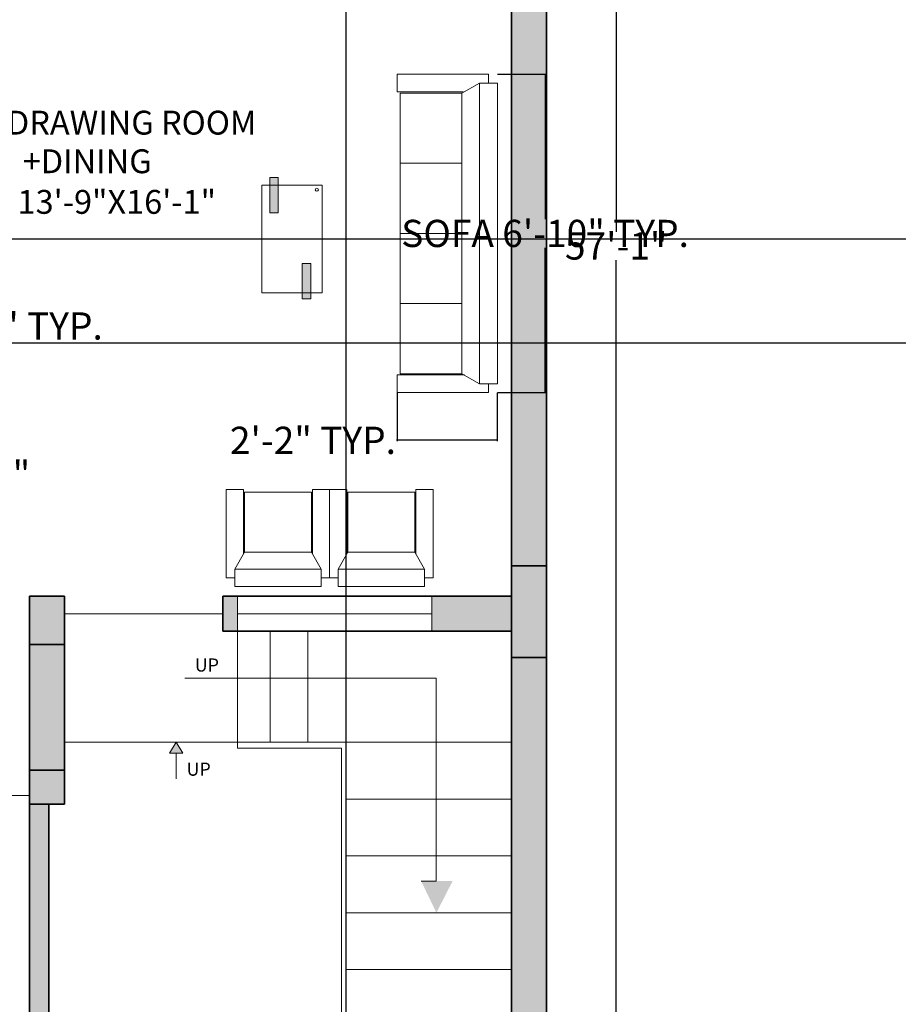
# Model space of a CAD drawing. Units: inches. Extents: x -17 to 892, y -721 to 172.
# Tile 3 of 11: x 212 to 438, y -462 to -209. Entities that reach past the tile are written whole.
import ezdxf

# ---------------------------------------------------------------- set-up
doc = ezdxf.new("R2010")
doc.units = ezdxf.units.IN
doc.header["$MEASUREMENT"] = 0
doc.layers.get('0').update_dxf_attribs({"color": 14})
for name, color, linetype, lineweight in [('A-ANNO-DIMS', 2, 'Continuous', 18), ('A-ANNO-SYMB', 7, 'Continuous', 18), ('A-AREA-IDEN', 7, 'Continuous', 18), ('A-COLS', 252, 'Continuous', 35), ('A-FLOR-STRS', 8, 'Continuous', 18), ('A-WALL-PATT', 14, 'Continuous', 13), ('doors', 4, 'Continuous', 18), ('furniture', 252, 'Continuous', 18), ('walls', 252, 'Continuous', 35), ('windows', 161, 'Continuous', 18)]:
    doc.layers.add(name, color=color, linetype=linetype, lineweight=lineweight)
doc.layers.add('A-COLS-PATT', color=254, linetype='Continuous', lineweight=13, true_color=0xd7ebd2)
doc.styles.get("Standard").update_dxf_attribs({"font": 'arial.ttf'})
doc.dimstyles.get("Standard").update_dxf_attribs({"dimtxt": 7, "dimasz": 0.18, "dimexe": 0.18, "dimexo": 0.0625, "dimgap": 0.09, "dimtad": 0, "dimtih": 1, "dimtoh": 1, "dimzin": 0, "dimdsep": 46, "dimlunit": 3, "dimtxsty": 'Standard', "dimcen": 0.09, "dimadec": 0, "dimazin": 0, "dimtfac": 1, "dimtofl": 0, "dimtmove": 0, "dimatfit": 3, "dimfxl": 1, "dimtolj": 1, "dimtzin": 0, "dimarcsym": 0})

# ---------------------------------------------------------------- blocks, each defined once
blk = doc.blocks.new('FABRIC SOFA 1S')
at = {"layer": 'furniture'}
for p, q in [((3, 18.12), (34, 18.12)), ((3, 15.12), (3, 18.12)), ((34, 12.12), (34, 18.12)), ((0, -15.12), (0, 15.12)), ((6, 15.12), (0, 15.12)), ((6, -15.12), (6, 15.12)), ((12, 11.75), (6, 15.12)), ((11.33, 12.12), (34, 12.12)), ((6, -15.12), (12, -11.75)), ((11.33, -12.12), (34, -12.12)), ((34, -12.12), (34, -18.12)), ((6, -15.12), (0, -15.12)), ((3, -18.12), (3, -15.12)), ((3, -18.12), (34, -18.12))]:
    blk.add_line(p, q, dxfattribs=at)
blk.add_lwpolyline([(12, -11.75), (12, 11.75), (33, 11.75), (33, -11.75)], close=True, dxfattribs=at)
blk = doc.blocks.new('FABRIC SOFA 4S')
at = {"layer": 'furniture'}
for p, q in [((3, 54), (34, 54)), ((3, 51), (3, 54)), ((34, 48), (34, 54)), ((0, -51), (0, 51)), ((6, 51), (0, 51)), ((6, -51), (6, 51)), ((12, 47.63), (6, 51)), ((11.14, 48), (34, 48)), ((33, 23.81), (12, 23.81)), ((33, 0), (12, 0)), ((33, -23.81), (12, -23.81)), ((6, -51), (12, -47.63)), ((11.54, -48), (34, -48)), ((34, -48), (34, -54)), ((6, -51), (0, -51)), ((3, -54), (3, -51)), ((3, -54), (34, -54))]:
    blk.add_line(p, q, dxfattribs=at)
blk.add_lwpolyline([(12, -47.63), (12, 47.63), (33, 47.63), (33, -47.63)], close=True, dxfattribs=at)
blk = doc.blocks.new('*D16')
at = {"layer": 'A-ANNO-DIMS', "color": 0, "lineweight": -2, "transparency": 16777216}
for p, q in [((364.49, 89.9), (365.24, 89.9)), ((365.06, 89.72), (365.06, -263.08)), ((365.06, -623.21), (365.06, -270.41)), ((364.49, -623.39), (365.24, -623.39))]:
    blk.add_line(p, q, dxfattribs=at)
at = {"layer": 'A-ANNO-DIMS', "color": 0, "lineweight": 100, "transparency": 16777216}
for points in [[(365.03, 89.72), (365.09, 89.72), (365.06, 89.9)], [(365.03, -623.21), (365.09, -623.21), (365.06, -623.39)]]:
    blk.add_solid(points, dxfattribs=at)
at = {"layer": 'Defpoints', "color": 0, "lineweight": 100, "transparency": 16777216}
for p in [(364.43, 89.9), (364.43, -623.39), (365.06, -623.39)]:
    blk.add_point(p, dxfattribs=at)
at = {"layer": 'A-ANNO-DIMS', "color": 0, "transparency": 16777216, "insert": (365.06, -266.74), "char_height": 7, "attachment_point": 5}
blk.add_mtext('\\A1;57\'-1"', dxfattribs=at)
blk = doc.blocks.new('TABLE-COCKTAIL')
h = blk.add_hatch(color=256)
h.dxf.hatch_style = 1
h.paths.add_polyline_path([(4.23, 29.31), (2.04, 29.31), (2.04, 22.19), (4.23, 22.19)])
h.paths.add_polyline_path([(4.23, 31.28), (2.04, 31.28), (2.04, 29.31), (4.23, 29.31)])
h.paths.add_polyline_path([(12.58, 9.09), (10.39, 9.09), (10.39, 1.62), (12.58, 1.62)])
h.paths.add_polyline_path([(12.58, 1.62), (10.39, 1.62), (10.39, 0), (12.58, 0)])
for p, q in [((2.04, 31.28), (4.23, 31.28)), ((2.04, 22.19), (2.04, 31.28)), ((4.23, 31.28), (4.23, 22.19)), ((0, 29.31), (0, 1.62)), ((15.53, 29.31), (0, 29.31)), ((15.53, 1.62), (15.53, 29.31)), ((4.23, 22.19), (2.04, 22.19)), ((10.39, 9.09), (12.58, 9.09)), ((10.39, 0), (10.39, 9.09)), ((12.58, 9.09), (12.58, 0)), ((0, 1.62), (15.53, 1.62)), ((12.58, 0), (10.39, 0))]:
    blk.add_line(p, q)
blk.add_circle((14.17, 28.1), 0.401)
blk = doc.blocks.new('STAIR-DIRECTION')
h = blk.add_hatch(color=256)
h.dxf.hatch_style = 1
h.paths.add_polyline_path([(64.68, 8.16), (60.81, 8.16), (64.68, 0.16)])
h.paths.add_polyline_path([(68.92, 8.16), (64.68, 8.16), (64.68, 0.16), (64.75, 0)])
for p, q in [((0, 60.33), (64.68, 60.33)), ((64.68, 60.33), (64.68, 8.16)), ((64.68, 8.16), (60.81, 8.16))]:
    blk.add_line(p, q)
blk = doc.blocks.new('*D44')
at = {"layer": 'A-ANNO-DIMS', "color": 0, "lineweight": -2, "transparency": 16777216}
for p, q in [((334.53, -222.56), (346.93, -222.56)), ((346.75, -222.74), (346.75, -259.8)), ((346.75, -304.28), (346.75, -267.22)), ((334.53, -304.46), (346.93, -304.46))]:
    blk.add_line(p, q, dxfattribs=at)
at = {"layer": 'A-ANNO-DIMS', "color": 0, "lineweight": 100, "transparency": 16777216}
for points in [[(346.72, -222.74), (346.78, -222.74), (346.75, -222.56)], [(346.72, -304.28), (346.78, -304.28), (346.75, -304.46)]]:
    blk.add_solid(points, dxfattribs=at)
at = {"layer": 'Defpoints', "color": 0, "lineweight": 100, "transparency": 16777216}
for p in [(334.46, -222.56), (334.46, -304.46), (346.75, -304.46)]:
    blk.add_point(p, dxfattribs=at)
at = {"layer": 'A-ANNO-DIMS', "color": 0, "transparency": 16777216, "insert": (346.75, -263.51), "char_height": 7, "attachment_point": 5}
blk.add_mtext('\\A1;SOFA 6\'-10" TYP.', dxfattribs=at)
blk = doc.blocks.new('*D45')
at = {"layer": 'A-ANNO-DIMS', "color": 0, "lineweight": -2, "transparency": 16777216}
for p, q in [((308.68, -304.52), (308.68, -316.93)), ((334.46, -304.52), (334.46, -316.93)), ((308.68, -316.75), (308.5, -316.75)), ((334.28, -316.75), (308.86, -316.75))]:
    blk.add_line(p, q, dxfattribs=at)
at = {"layer": 'A-ANNO-DIMS', "color": 0, "lineweight": 100, "transparency": 16777216}
for points in [[(308.86, -316.72), (308.86, -316.78), (308.68, -316.75)], [(334.28, -316.72), (334.28, -316.78), (334.46, -316.75)]]:
    blk.add_solid(points, dxfattribs=at)
at = {"layer": 'Defpoints', "color": 0, "lineweight": 100, "transparency": 16777216}
for p in [(308.68, -304.46), (334.46, -304.46), (308.68, -316.75)]:
    blk.add_point(p, dxfattribs=at)
at = {"layer": 'A-ANNO-DIMS', "color": 0, "transparency": 16777216, "insert": (287.02, -316.75), "char_height": 7, "attachment_point": 5}
blk.add_mtext('\\A1;2\'-2" TYP.', dxfattribs=at)
blk = doc.blocks.new('*D51')
at = {"layer": 'A-ANNO-DIMS', "color": 0, "lineweight": -2, "transparency": 16777216}
for p, q in [((170.93, -291.56), (170.93, -287.14)), ((171.11, -287.32), (173.4, -287.32)), ((173.58, -291.56), (173.58, -287.14)), ((173.58, -287.32), (173.76, -287.32))]:
    blk.add_line(p, q, dxfattribs=at)
at = {"layer": 'A-ANNO-DIMS', "color": 0, "lineweight": 100, "transparency": 16777216}
for points in [[(171.11, -287.29), (171.11, -287.35), (170.93, -287.32)], [(173.4, -287.29), (173.4, -287.35), (173.58, -287.32)]]:
    blk.add_solid(points, dxfattribs=at)
at = {"layer": 'Defpoints', "color": 0, "lineweight": 100, "transparency": 16777216}
for p in [(173.58, -287.32), (170.93, -291.63), (173.58, -291.63)]:
    blk.add_point(p, dxfattribs=at)
at = {"layer": 'A-ANNO-DIMS', "color": 0, "transparency": 16777216, "insert": (203.34, -287.32), "char_height": 7, "attachment_point": 5}
blk.add_mtext('\\A1;0\'-2 1/2" TYP.', dxfattribs=at)
blk = doc.blocks.new('*D54')
at = {"layer": 'A-ANNO-DIMS', "color": 0, "lineweight": -2, "transparency": 16777216}
for p, q in [((133.16, -328.67), (133.16, -325.31)), ((133.34, -325.49), (154.58, -325.49)), ((154.76, -328.67), (154.76, -325.31)), ((154.76, -325.49), (154.94, -325.49))]:
    blk.add_line(p, q, dxfattribs=at)
at = {"layer": 'A-ANNO-DIMS', "color": 0, "lineweight": 100, "transparency": 16777216}
for points in [[(133.34, -325.46), (133.34, -325.52), (133.16, -325.49)], [(154.58, -325.46), (154.58, -325.52), (154.76, -325.49)]]:
    blk.add_solid(points, dxfattribs=at)
at = {"layer": 'Defpoints', "color": 0, "lineweight": 100, "transparency": 16777216}
for p in [(154.76, -325.49), (133.16, -328.73), (154.76, -328.73)]:
    blk.add_point(p, dxfattribs=at)
at = {"layer": 'A-ANNO-DIMS', "color": 0, "transparency": 16777216, "insert": (184.26, -325.49), "char_height": 7, "attachment_point": 5}
blk.add_mtext('\\A1;HOB 1\'-9 1/2"', dxfattribs=at)
blk = doc.blocks.new('*D61')
at = {"layer": 'A-ANNO-DIMS', "color": 0, "lineweight": -2, "transparency": 16777216}
for p, q in [((170.99, -264.92), (841.36, -264.92)), ((841.18, -265.1), (841.18, -274.56)), ((841.18, -291.45), (841.18, -281.98)), ((170.99, -291.63), (841.36, -291.63))]:
    blk.add_line(p, q, dxfattribs=at)
at = {"layer": 'A-ANNO-DIMS', "color": 0, "lineweight": 100, "transparency": 16777216}
for points in [[(841.15, -265.1), (841.21, -265.1), (841.18, -264.92)], [(841.15, -291.45), (841.21, -291.45), (841.18, -291.63)]]:
    blk.add_solid(points, dxfattribs=at)
at = {"layer": 'Defpoints', "color": 0, "lineweight": 100, "transparency": 16777216}
for p in [(170.93, -264.92), (170.93, -291.63), (841.18, -291.63)]:
    blk.add_point(p, dxfattribs=at)
at = {"layer": 'A-ANNO-DIMS', "color": 0, "transparency": 16777216, "insert": (841.18, -278.27), "char_height": 7, "attachment_point": 5}
blk.add_mtext('\\A1;2\'-2 1/2"', dxfattribs=at)
blk = doc.blocks.new('*D63')
at = {"layer": 'A-ANNO-DIMS', "color": 0, "lineweight": -2, "transparency": 16777216}
for p, q in [((295.55, -619.99), (295.55, 161.84)), ((295.73, 161.66), (299.27, 161.66)), ((337.9, 161.66), (334.36, 161.66)), ((338.08, -619.99), (338.08, 161.84))]:
    blk.add_line(p, q, dxfattribs=at)
at = {"layer": 'A-ANNO-DIMS', "color": 0, "lineweight": 100, "transparency": 16777216}
for points in [[(295.73, 161.69), (295.73, 161.63), (295.55, 161.66)], [(337.9, 161.69), (337.9, 161.63), (338.08, 161.66)]]:
    blk.add_solid(points, dxfattribs=at)
at = {"layer": 'Defpoints', "color": 0, "lineweight": 100, "transparency": 16777216}
for p in [(338.08, 161.66), (295.55, -620.06), (338.08, -620.06)]:
    blk.add_point(p, dxfattribs=at)
at = {"layer": 'A-ANNO-DIMS', "color": 0, "transparency": 16777216, "insert": (316.82, 161.66), "char_height": 7, "attachment_point": 5}
blk.add_mtext('\\A1;3\'-6 1/2"', dxfattribs=at)

msp = doc.modelspace()

# ---------------------------------------------------------------- hatches: boundary and pattern name
at = {"layer": 'A-ANNO-SYMB'}
h = msp.add_hatch(color=256, dxfattribs=at)
h.dxf.hatch_style = 1
h.paths.add_polyline_path([(251.822, -394.434), (250.105, -397.283), (251.822, -397.283), (253.554, -397.283)])
at = {"layer": 'A-COLS-PATT'}
h = msp.add_hatch(color=256, dxfattribs=at)
h.dxf.hatch_style = 1
h.paths.add_polyline_path([(92.084, 61.611), (83.084, 61.611), (83.084, 43.692), (92.084, 43.692)])
h.paths.add_polyline_path([(347.084, 61.611), (338.084, 61.611), (338.084, 43.692), (347.084, 43.692)])
h.paths.add_polyline_path([(222.053, 61.611), (209.95, 61.611), (209.95, 52.611), (222.053, 52.611)])
h.paths.add_polyline_path([(284.798, 61.611), (274.584, 61.611), (274.584, 52.611), (284.798, 52.611)])
h.paths.add_polyline_path([(223.084, -106.389), (214.084, -106.389), (214.084, -119.959), (223.084, -119.959)])
h.paths.add_polyline_path([(347.084, -148.653), (338.084, -148.653), (338.084, -172.24), (347.084, -172.24)])
h.paths.add_polyline_path([(92.084, -102.402), (83.084, -102.402), (83.084, -119.959), (92.084, -119.959)])
h.paths.add_polyline_path([(92.084, -205.889), (83.084, -205.889), (83.084, -216.319), (92.084, -216.319)])
h.paths.add_polyline_path([(347.084, -349.073), (338.084, -349.073), (338.084, -372.66), (347.084, -372.66)])
h.paths.add_polyline_path([(347.084, -610.134), (338.084, -610.134), (338.084, -614.389), (338.084, -623.342), (347.084, -623.342)])
h.paths.add_polyline_path([(221.166, -610.357), (214.084, -610.357), (214.084, -623.389), (219.084, -623.389), (221.166, -623.389), (221.166, -621.723)])
h.paths.add_polyline_path([(90.166, -610.357), (83.084, -610.357), (83.084, -623.389), (90.166, -623.389)])
h.paths.add_polyline_path([(223.084, -401.64), (214.084, -401.64), (214.084, -410.389), (223.084, -410.389)])
h.paths.add_polyline_path([(223.084, -356.889), (214.084, -356.889), (214.084, -369.273), (223.084, -369.273)])
h.paths.add_polyline_path([(92.084, -398.492), (83.084, -398.492), (83.084, -410.389), (92.084, -410.389)])
h.paths.add_polyline_path([(92.084, -348.918), (83.084, -348.918), (83.084, -360.706), (92.084, -360.706)])
at = {"layer": 'A-WALL-PATT'}
h = msp.add_hatch(color=256, dxfattribs=at)
h.dxf.hatch_style = 1
h.paths.add_polyline_path([(111.26, 61.611), (92.084, 61.611), (92.084, 52.611), (111.26, 52.611)])
h.paths.add_polyline_path([(209.95, 61.611), (179.154, 61.611), (179.154, 52.611), (209.95, 52.611)])
h.paths.add_polyline_path([(338.084, 61.611), (284.798, 61.611), (284.798, 52.611), (338.084, 52.611)])
h.paths.add_polyline_path([(279.084, 23.861), (274.584, 23.861), (274.584, -0.389), (279.084, -0.389)])
h.paths.add_polyline_path([(279.084, 52.611), (274.584, 52.611), (274.584, 46.881), (276.834, 46.881), (279.084, 46.881)])
h.paths.add_polyline_path([(279.084, -0.389), (274.584, -0.389), (274.584, -4.889), (279.084, -4.889)])
h.paths.add_polyline_path([(304.22, -0.389), (279.084, -0.389), (279.084, -4.889), (304.22, -4.889)])
h.paths.add_polyline_path([(347.084, 43.692), (338.084, 43.692), (338.084, -148.653), (347.084, -148.653)])
h.paths.add_polyline_path([(338.084, -154.889), (264.103, -154.889), (264.103, -163.889), (338.084, -163.889)])
h.paths.add_polyline_path([(223.084, -119.959), (214.084, -119.959), (214.084, -163.889), (223.084, -163.889)])
h.paths.add_polyline_path([(218.584, 52.611), (214.084, 52.611), (214.084, -106.389), (218.584, -106.389)])
h.paths.add_polyline_path([(92.084, -8.943), (83.084, -8.943), (83.084, -49.69), (87.584, -49.69), (92.084, -49.69)])
h.paths.add_polyline_path([(92.084, 43.692), (83.084, 43.692), (83.084, 33.018), (87.584, 33.018), (92.084, 33.018)])
h.paths.add_polyline_path([(92.084, -91.651), (83.084, -91.651), (83.084, -102.402), (92.084, -102.402)])
h.paths.add_polyline_path([(92.084, -119.959), (83.084, -119.959), (83.084, -151.855), (87.584, -151.855), (92.084, -151.855)])
h.paths.add_polyline_path([(173.584, -108.639), (173.584, -106.389), (173.084, -106.389), (92.084, -106.389), (92.084, -110.889), (169.084, -110.889), (169.084, -176.029), (173.584, -176.029)])
h.paths.add_polyline_path([(92.084, -185.221), (83.084, -185.221), (83.084, -205.889), (92.084, -205.889)])
h.paths.add_polyline_path([(92.084, -216.319), (83.084, -216.319), (83.084, -259.015), (87.584, -259.015), (92.084, -259.015)])
h.paths.add_polyline_path([(173.584, -205.889), (92.084, -205.889), (92.084, -210.389), (169.084, -210.389), (169.084, -236.193), (173.584, -236.193)])
h.paths.add_polyline_path([(92.084, -300.976), (83.084, -300.976), (83.084, -348.918), (92.084, -348.918)])
h.paths.add_polyline_path([(87.584, -410.389), (83.084, -410.389), (83.084, -610.357), (87.584, -610.357)])
h.paths.add_polyline_path([(115.523, -614.389), (90.166, -614.389), (90.166, -623.389), (115.523, -623.389)])
h.paths.add_polyline_path([(214.084, -614.389), (174.149, -614.389), (174.149, -623.389), (214.084, -623.389)])
h.paths.add_polyline_path([(219.084, -410.389), (214.084, -410.389), (214.084, -610.357), (219.084, -610.357)])
h.paths.add_polyline_path([(347.084, -372.66), (338.084, -372.66), (338.084, -610.134), (347.084, -610.134)])
h.paths.add_polyline_path([(347.084, -172.24), (338.084, -172.24), (338.084, -349.073), (347.084, -349.073)])
h.paths.add_polyline_path([(338.084, -356.889), (317.618, -356.889), (317.618, -365.889), (338.084, -365.889)])
h.paths.add_polyline_path([(267.632, -356.889), (263.828, -356.889), (263.828, -365.889), (267.632, -365.889)])
h.paths.add_polyline_path([(223.084, -369.273), (214.084, -369.273), (214.084, -401.64), (223.084, -401.64)])

# ---------------------------------------------------------------- linework, layer by layer
at = {"layer": 'A-ANNO-SYMB'}
for p, q in [((251.822, -394.434), (250.105, -397.283)), ((253.554, -397.283), (251.822, -394.434)), ((250.105, -397.283), (251.822, -397.283)), ((251.822, -397.283), (253.554, -397.283)), ((251.822, -397.283), (251.822, -403.838))]:
    msp.add_line(p, q, dxfattribs=at)
at = {"layer": 'A-COLS'}
for p, q in [((338.084, -349.073), (347.084, -349.073)), ((214.084, -356.889), (223.084, -356.889)), ((214.084, -369.273), (223.084, -369.273)), ((338.084, -372.66), (347.084, -372.66)), ((214.084, -401.64), (223.084, -401.64)), ((214.084, -410.389), (223.084, -410.389))]:
    msp.add_line(p, q, dxfattribs=at)
at = {"layer": 'A-FLOR-STRS'}
for p, q in [((267.632, -365.889), (267.632, -395.993)), ((276.034, -365.889), (276.034, -394.434)), ((285.71, -365.889), (285.71, -394.434)), ((295.55, -365.889), (295.55, -394.434)), ((223.084, -394.434), (295.55, -394.434)), ((295.55, -394.434), (295.55, -620.057)), ((295.55, -394.434), (338.084, -394.434)), ((267.632, -395.993), (294.357, -395.993)), ((294.357, -395.993), (294.357, -564.936)), ((295.55, -409.063), (338.084, -409.063)), ((295.55, -423.692), (338.084, -423.692)), ((295.55, -438.321), (338.084, -438.321)), ((295.55, -452.95), (338.084, -452.95))]:
    msp.add_line(p, q, dxfattribs=at)
at = {"layer": 'doors'}
for p, q in [((263.828, -361.389), (223.084, -361.389)), ((173.584, -408.139), (214.084, -408.139))]:
    msp.add_line(p, q, dxfattribs=at)
at = {"layer": 'walls'}
for p, q in [((338.084, 61.611), (338.084, -614.389)), ((347.084, 61.611), (347.084, -623.389)), ((214.084, -623.389), (214.084, -356.889)), ((223.084, -410.389), (223.084, -356.889)), ((263.828, -356.889), (263.828, -365.889)), ((263.828, -356.889), (338.084, -356.889)), ((263.828, -365.889), (263.828, -365.889)), ((263.828, -365.889), (338.084, -365.889)), ((219.084, -610.357), (219.084, -410.389))]:
    msp.add_line(p, q, dxfattribs=at)
at = {"layer": 'windows'}
for p, q in [((267.632, -356.889), (267.632, -365.889)), ((317.618, -356.889), (267.632, -356.889)), ((267.632, -356.889), (267.632, -361.389)), ((317.618, -365.889), (317.618, -356.889)), ((267.632, -361.389), (317.618, -361.389)), ((267.632, -365.889), (317.618, -365.889))]:
    msp.add_line(p, q, dxfattribs=at)

# ---------------------------------------------------------------- block references
at = {"layer": 'A-ANNO-SYMB'}
msp.add_blockref('STAIR-DIRECTION', (254.041, -438.321), dxfattribs=at)
at = {"layer": 'furniture'}
for name, p, xscale, yscale, zscale, rotation in [('FABRIC SOFA 4S', (334.465, -263.508), 0.7583822975527559, 0.7583822975527559, 0.7583822975527559, 180), ('FABRIC SOFA 1S', (278.017, -354.335), 0.7339463821036302, 0.7339463821036302, 0.7339463821036302, 90.00000000000087), ('FABRIC SOFA 1S', (304.622, -354.335), 0.7339463821036302, 0.7339463821036302, 0.7339463821036302, 90)]:
    msp.add_blockref(name, p, dxfattribs=dict(at, xscale=xscale, yscale=yscale, zscale=zscale, rotation=rotation))
msp.add_blockref('TABLE-COCKTAIL', (273.858, -280.375), dxfattribs=at)

# ---------------------------------------------------------------- texts
at = {"layer": 'A-ANNO-SYMB'}
for p in [(256.619, -376.252), (254.499, -403.06)]:
    msp.add_text('UP', height=3.3722, dxfattribs=at).set_placement(p)
at = {"layer": 'A-AREA-IDEN'}
for s, p in [('DRAWING ROOM', (208.262, -238.074)), ('+DINING', (212.346, -248.01)), ('13\'-9"X16\'-1"', (211.017, -258.463))]:
    msp.add_text(s, height=6.1361, dxfattribs=at).set_placement(p)

# ---------------------------------------------------------------- dimensions: what is measured, and where the dimension line sits
at = {"layer": 'A-ANNO-DIMS'}
dim = msp.add_linear_dim(base=(338.084, 161.663), p1=(295.55, -620.057), p2=(338.084, -620.057), dimstyle='Standard', override={"dimdec": 1, "dimlfac": 1, "dimrnd": 0, "dimzin": 1, "dimdsep": 46, "dimlunit": 4, "dimfrac": 2}, dxfattribs=at)
dim.commit()
dim.dimension.update_dxf_attribs({"geometry": '*D63', "text_midpoint": (316.817, 161.663)})
for base, p1, p2, angle, text, override, picture, middle in [((365.057, -623.389), (364.432, 89.902), (364.432, -623.389), 90, '57\'-1"', {"dimclrd": 0, "dimclre": 0, "dimclrt": 0}, '*D16', (365.057, -266.744)), ((346.75, -304.461), (334.465, -222.556), (334.465, -304.461), 270, 'SOFA <> TYP.', {"dimdec": 1, "dimlfac": 1, "dimrnd": 0, "dimzin": 1, "dimdsep": 46, "dimlunit": 4, "dimfrac": 2}, '*D44', (346.75, -263.508)), ((308.68, -316.747), (334.465, -304.461), (308.68, -304.461), 180, '<> TYP.', {"dimdec": 1, "dimlfac": 1, "dimrnd": 0, "dimzin": 1, "dimdsep": 46, "dimlunit": 4, "dimfrac": 2}, '*D45', (287.016, -316.747))]:
    dim = msp.add_linear_dim(base=base, p1=p1, p2=p2, angle=angle, text=text, dimstyle='Standard', override=override, dxfattribs=at)
    dim.commit()
    dim.dimension.update_dxf_attribs({"geometry": picture, "text_midpoint": middle})
dim = msp.add_linear_dim(base=(841.176, -291.625), p1=(170.932, -264.917), p2=(170.932, -291.625), angle=90, dimstyle='Standard', override={"dimdec": 1, "dimlfac": 1, "dimrnd": 0, "dimzin": 1, "dimdsep": 46, "dimlunit": 4, "dimfrac": 2}, dxfattribs=at)
dim.commit()
dim.dimension.update_dxf_attribs({"geometry": '*D61', "text_midpoint": (841.176, -278.271)})
for base, p1, p2, text, picture, middle in [((173.584, -287.316), (170.932, -291.625), (173.584, -291.625), '<> TYP.', '*D51', (203.344, -287.316)), ((154.762, -325.488), (133.162, -328.728), (154.762, -328.728), 'HOB <>', '*D54', (184.256, -325.488))]:
    dim = msp.add_linear_dim(base=base, p1=p1, p2=p2, text=text, dimstyle='Standard', override={"dimdec": 1, "dimlfac": 1, "dimrnd": 0, "dimzin": 1, "dimdsep": 46, "dimlunit": 4, "dimfrac": 2}, dxfattribs=at)
    dim.commit()
    dim.dimension.update_dxf_attribs({"geometry": picture, "text_midpoint": middle})

doc.saveas('drawing.dxf')
